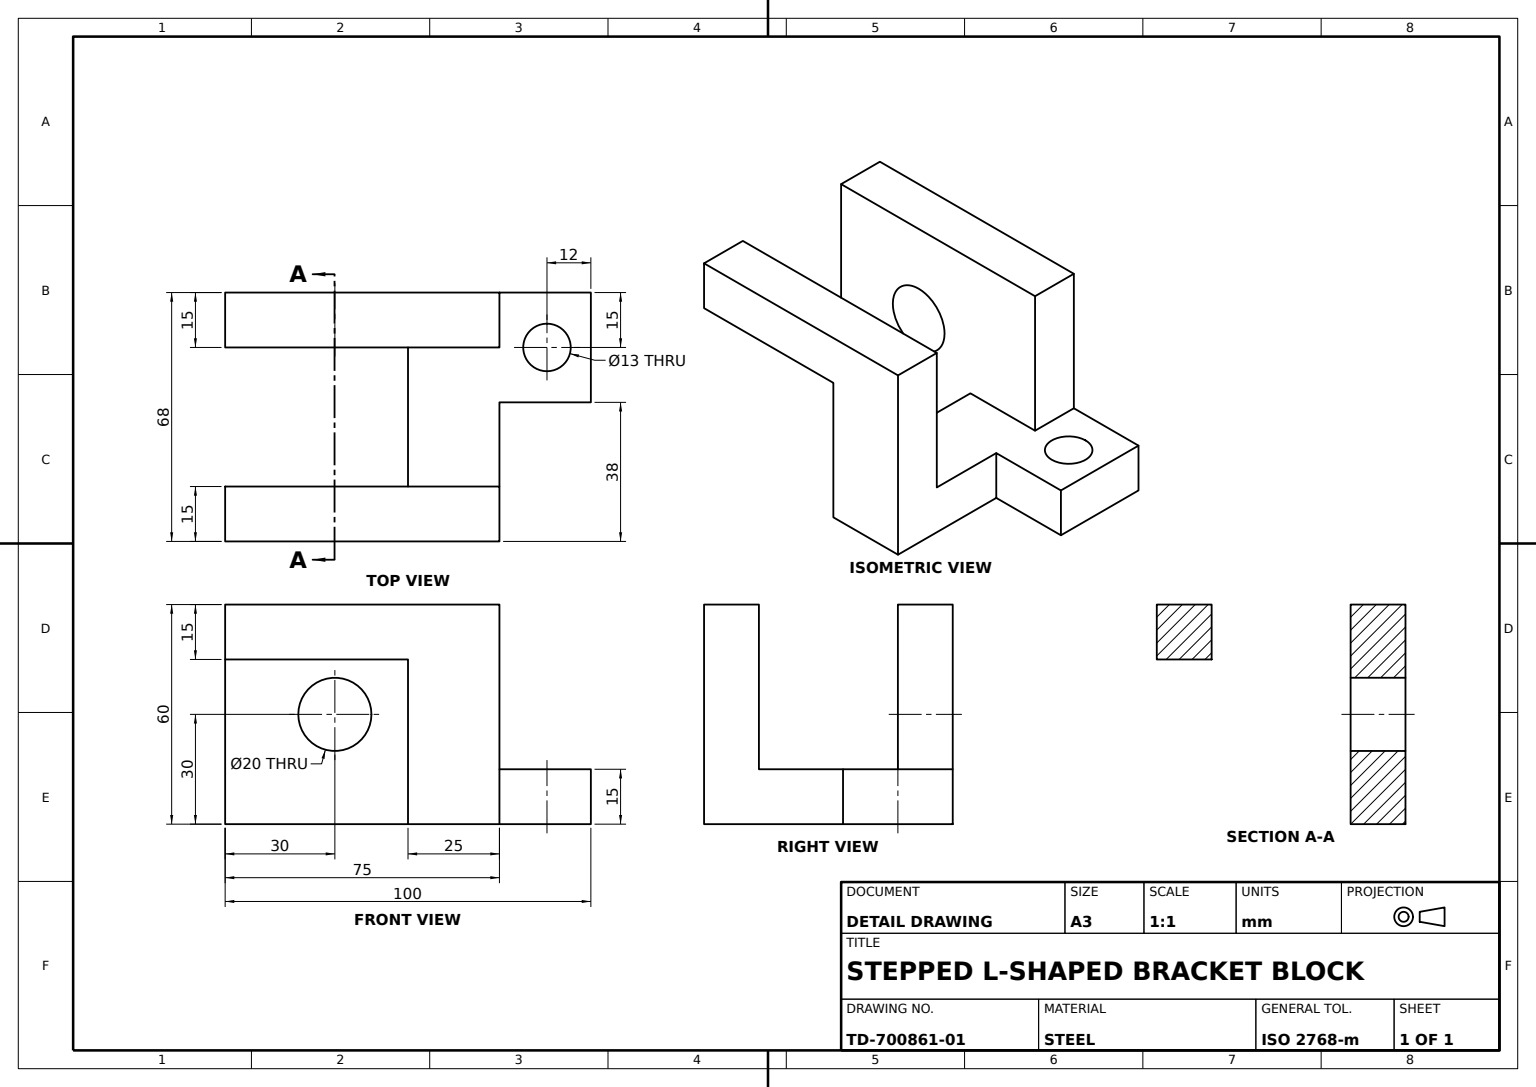
SolidWorks part; units mm, degrees
material "Plain Carbon Steel"
ref_plane "Front Plane" through (0, 0, 0) normal (0, 0, 1) x (1, 0, 0)
ref_plane "Top Plane" through (0, 0, 0) normal (0, 1, 0) x (1, 0, 0)
ref_plane "Right Plane" through (0, 0, 0) normal (1, 0, 0) x (0, 0, -1)
sketch "L Side Wall Sketch" plane through (0, 0, 0) normal (0, 0, 1) x (1, 0, 0)
  line L0 (0, 0) -> (0, 60)
  line L1 (0, 60) -> (-75, 60)
  line L2 (-75, 60) -> (-75, 45)
  line L3 (-75, 45) -> (-25, 45)
  line L4 (-25, 45) -> (-25, 0)
  line L5 (-25, 0) -> (0, 0)
  dimension "D1" = 75
  dimension "D2" = 15
  dimension "D3" = 60
  dimension "D4" = 25
extrude "L Side Wall" add sketch "L Side Wall Sketch" against normal blind 15
sketch "Base Flange Sketch" plane through (0, 0, 0) normal (0, 1, 0) x (1, 0, 0)
  line L0 (-25, 53) -> (0, 53)
  line L1 (0, 0) -> (-25, 0)
  line L2 (0, 0) -> (0, 38)
  line L4 (-25, 0) -> (-25, 53)
  line L5 (0, 68) -> (25, 68)
  line L6 (0, 68) -> (0, 53)
  line L7 (0, 38) -> (25, 38)
  line L8 (25, 68) -> (25, 38)
  line L9 (0, 15) -> (-75, 15) construction
  line L10 (0, 53) -> (0, 68)
  dimension "D1" = 15
  dimension "D2" = 68
  dimension "D3" = 23
  dimension "D4" = 25
  dimension "D5" = 25
  dimension "D6" = 30
  dimension "D7" = 38
extrude "Base Flange With Tab" add sketch "Base Flange Sketch" along normal blind 15 contours L8 L5 L6 L0 L4 L1 L2 L7
sketch "Upright Plate Sketch" plane through (0, 0, 0) normal (0, 1, 0) x (1, 0, 0)
  line L0 (0, 68) -> (25, 68) construction
  line L1 (0, 68) -> (-75, 68)
  line L2 (0, 68) -> (0, 53)
  line L3 (0, 53) -> (-75, 53)
  line L4 (-75, 68) -> (-75, 53)
  dimension "D1" = 15
  dimension "D2" = 75
extrude "Upright Plate" add sketch "Upright Plate Sketch" along normal blind 60
sketch "Upright Cross Hole Sketch" plane through (0, 0, -68) normal (0, 0, -1) x (-1, 0, 0)
  line L0 (75, 60) -> (75, 0) construction
  line L1 (75, 0) -> (-25, 0) construction
  circle A0 centre (45, 30) radius 10
  dimension "D3" = 20
  dimension "D1" = 30
  dimension "D2" = 30
extrude "Upright Cross Hole" cut sketch "Upright Cross Hole Sketch" against normal through all
sketch "Tab Mounting Hole Sketch" plane through (0, 15, 0) normal (0, 1, 0) x (1, 0, 0)
  line L0 (25, 68) -> (25, 38) construction
  line L1 (0, 68) -> (25, 68) construction
  circle A0 centre (13, 53) radius 6.5
  dimension "D1" = 13
  dimension "D2" = 12
  dimension "D3" = 15
extrude "Tab Mounting Hole" cut sketch "Tab Mounting Hole Sketch" against normal through all both and the other way through all
